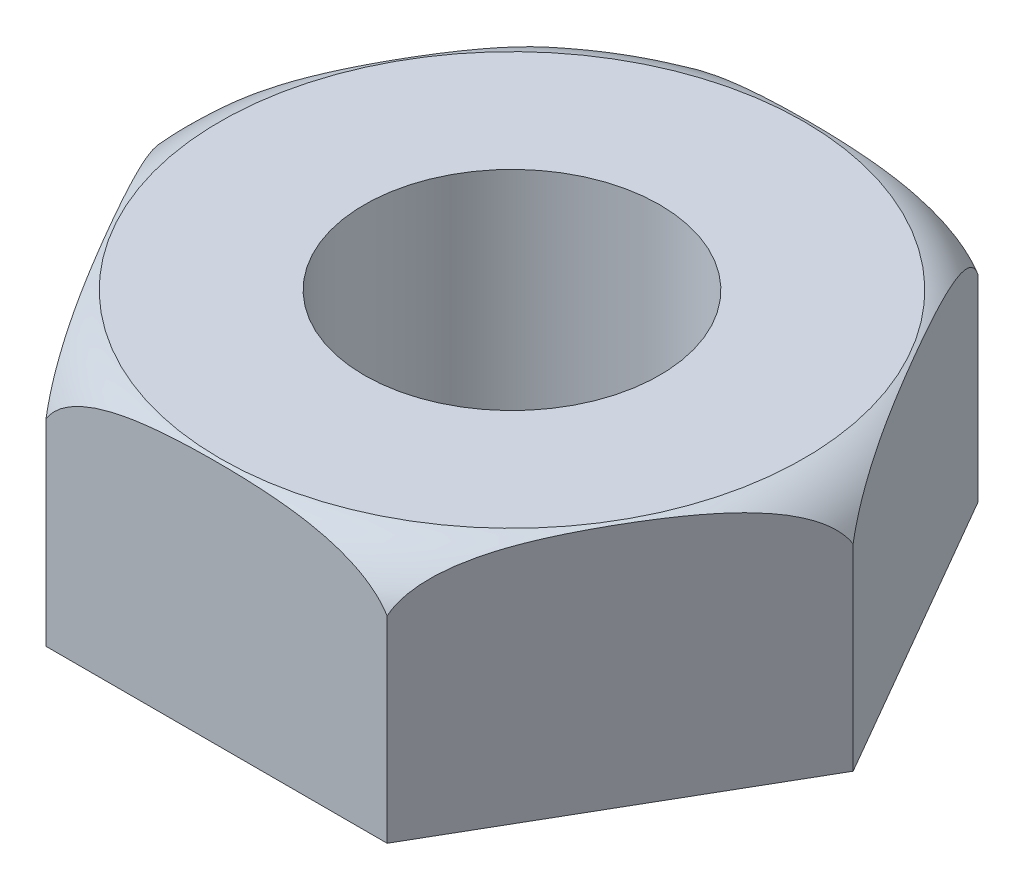
SolidWorks part; units mm, degrees
material "Plain Carbon Steel"
ref_plane "Front Plane" through (0, 0, 0) normal (0, 0, 1) x (1, 0, 0)
ref_plane "Top Plane" through (0, 0, 0) normal (0, 1, 0) x (1, 0, 0)
ref_plane "Right Plane" through (0, 0, 0) normal (1, 0, 0) x (0, 0, -1)
sketch "Hex Profile Sketch" plane through (0, 0, 0) normal (0, 1, 0) x (1, 0, 0)
  line L1 (13.8564, 0) -> (6.9282, 12)
  line L2 (6.9282, 12) -> (-6.9282, 12)
  line L3 (-6.9282, 12) -> (-13.8564, 0)
  line L4 (-13.8564, 0) -> (-6.9282, -12)
  line L5 (-6.9282, -12) -> (6.9282, -12)
  line L6 (6.9282, -12) -> (13.8564, 0)
  circle A0 centre (0, 0) radius 12 construction
  circle A1 centre (0, 0) radius 6
  dimension "D1" = 24
  dimension "D2" = 12
extrude "Hex Nut Body" add sketch "Hex Profile Sketch" along normal mid plane 10
sketch "Corner Chamfer Profile Sketch" plane through (0, 0, 0) normal (0, 0, 1) x (1, 0, 0)
  line L0 (0, -7.5191) -> (0, 8.148) construction
  line L1 (6.9282, 5) -> (13.8564, 5) construction
  line L2 (13.8564, 5) -> (13.8564, -5) construction
  line L3 (11.8564, 5) -> (13.8564, 5)
  line L4 (13.8564, 5) -> (13.8564, 3)
  arc A0 (11.8564, 5) -> (13.8564, 3) centre (10.9856, 2.1292) cw
  dimension "D1" = 3
  dimension "D2" = 2
  dimension "D3" = 2
revolve "Hex Corner Chamfer" cut sketch "Corner Chamfer Profile Sketch" angle 360 about L0
